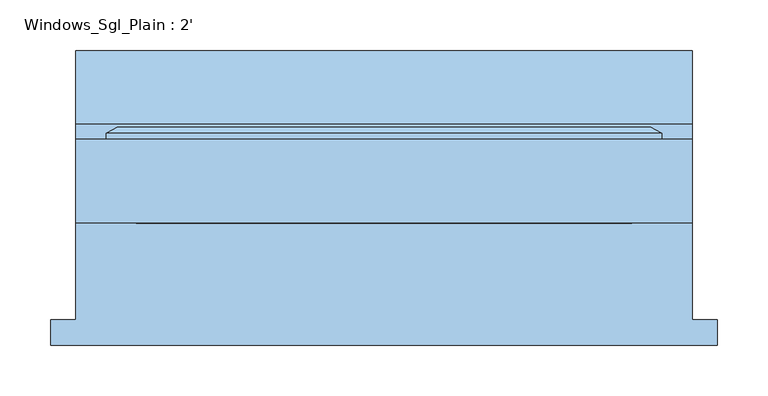
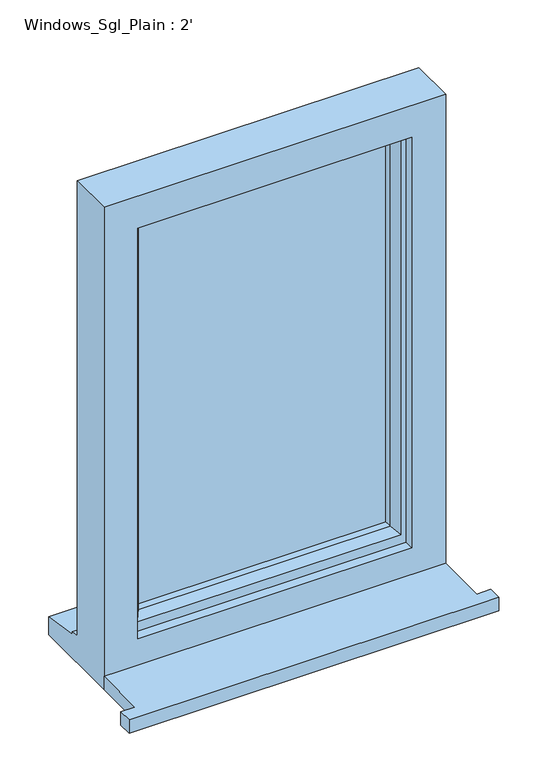
"""IFC4 building model written with IfcOpenShell, lengths in millimetres: window geometry, Windows_Sgl_Plain : 2'."""

from ifc_helpers import new_model, si_unit, frame, origin, place, context, project, spatial, polyline, outline, extrude, faceted_brep, source, transform, mapped, element, save


def windows_sgl_plain_2_8d1346b0(model_context):
    return source(origin(), model_context, "Body", "SolidModel", [
        extrude(outline(polyline([(-329.8, -130.8434322), (-329.8, -105.8434322), (-304.8, -105.8434322), (-304.8, -10.2434322), (304.8, -10.2434322), (304.8, -105.8434322), (329.8, -105.8434322), (329.8, -130.8434322), (-329.8, -130.8434322)])), frame((0.0, 0.0, 1200.0), z_axis=(0.0, 0.0, 1.0), x_axis=(1.0, 0.0, 0.0)), (0.0, 0.0, 1.0), 25.0),
        faceted_brep([(-304.8, -10.2434322, 1200.0), (304.8, -10.2434322, 1200.0), (304.8, -10.2434322, 2110.0), (-304.8, -10.2434322, 2110.0), (-244.8, -10.2434322, 2050.0), (244.8, -10.2434322, 2050.0), (244.8, -10.2434322, 1275.0), (-244.8, -10.2434322, 1275.0), (-304.8, 72.7565678, 2110.0), (-304.8, 72.7565678, 1251.0), (-304.8, 87.7565678, 1249.68767), (-304.8, 87.7565678, 1244.7449676), (-304.8, 160.2565678, 1233.8088847), (-304.8, 160.2565678, 1200.0), (304.8, 72.7565678, 2110.0), (304.8, 72.7565678, 1251.0), (-264.8, 72.7565678, 2070.0), (-264.8, 72.7565678, 1263.0), (264.8, 72.7565678, 1263.0), (264.8, 72.7565678, 2070.0), (-264.8, 7.7565678, 2070.0), (-264.8, 7.7565678, 1263.0), (264.8, 7.7565678, 2070.0), (264.8, 7.7565678, 1263.0), (-244.8, 7.7565678, 2050.0), (-244.8, 7.7565678, 1275.0), (244.8, 7.7565678, 1275.0), (244.8, 7.7565678, 2050.0), (304.8, 160.2565678, 1200.0), (304.8, 160.2565678, 1233.8088847), (304.8, 87.7565678, 1244.7449676), (304.8, 87.7565678, 1249.68767)], [[[0, 1, 2, 3], [4, 5, 6, 7]], [[0, 3, 8, 9, 10, 11, 12, 13]], [[9, 8, 14, 15], [16, 17, 18, 19]], [[17, 16, 20, 21]], [[20, 22, 23, 21], [24, 25, 26, 27]], [[24, 4, 7, 25]], [[3, 2, 14, 8]], [[16, 19, 22, 20]], [[5, 4, 24, 27]], [[15, 14, 2, 1, 28, 29, 30, 31]], [[19, 18, 23, 22]], [[5, 27, 26, 6]], [[28, 1, 0, 13]], [[29, 28, 13, 12]], [[30, 29, 12, 11]], [[31, 30, 11, 10]], [[15, 31, 10, 9]], [[21, 23, 18, 17]], [[7, 6, 26, 25]]]),
        extrude(outline(polyline([(234.8, 36.7565678), (-234.8, 36.7565678), (-234.8, 60.7565678), (234.8, 60.7565678), (234.8, 36.7565678)])), frame((0.0, 0.0, 1293.0), z_axis=(0.0, 0.0, 1.0), x_axis=(1.0, 0.0, 0.0)), (0.0, 0.0, 1.0), 747.0),
        faceted_brep([(-274.8, 72.7565678, 2080.0), (-274.8, 78.5300705, 2080.0), (-274.8, 78.5300705, 1253.0), (-274.8, 72.7565678, 1253.0), (-264.8, 7.7565678, 2070.0), (-264.8, 72.7565678, 2070.0), (-264.8, 72.7565678, 1263.0), (-264.8, 7.7565678, 1263.0), (-224.8, 22.2494677, 2030.0), (-234.9480377, 7.7565678, 2040.1480377), (-234.9480377, 7.7565678, 1292.8519623), (-224.8, 22.2494677, 1303.0), (-224.8, 36.7565678, 2030.0), (-224.8, 36.7565678, 1303.0), (-234.8, 60.7565678, 2040.0), (-234.8, 36.7565678, 2040.0), (-234.8, 36.7565678, 1293.0), (-234.8, 60.7565678, 1293.0), (-224.8, 78.5300705, 2030.0), (-224.8, 60.7565678, 2030.0), (-224.8, 60.7565678, 1303.0), (-224.8, 78.5300705, 1303.0), (-242.2457548, 84.3035732, 2047.4457548), (-242.2457548, 84.3035732, 1285.5542452), (-264.0153903, 84.3035732, 2069.2153903), (-264.0153903, 84.3035732, 1263.7846097), (274.8, 78.5300705, 1253.0), (274.8, 72.7565678, 1253.0), (264.8, 72.7565678, 1263.0), (264.8, 7.7565678, 1263.0), (234.9480377, 7.7565678, 1292.8519623), (224.8, 22.2494677, 1303.0), (224.8, 36.7565678, 1303.0), (234.8, 36.7565678, 1293.0), (234.8, 60.7565678, 1293.0), (224.8, 60.7565678, 1303.0), (224.8, 78.5300705, 1303.0), (242.2457548, 84.3035732, 1285.5542452), (264.0153903, 84.3035732, 1263.7846097), (274.8, 78.5300705, 2080.0), (274.8, 72.7565678, 2080.0), (264.8, 72.7565678, 2070.0), (264.8, 7.7565678, 2070.0), (234.9480377, 7.7565678, 2040.1480377), (224.8, 22.2494677, 2030.0), (224.8, 36.7565678, 2030.0), (234.8, 36.7565678, 2040.0), (234.8, 60.7565678, 2040.0), (224.8, 60.7565678, 2030.0), (224.8, 78.5300705, 2030.0), (242.2457548, 84.3035732, 2047.4457548), (264.0153903, 84.3035732, 2069.2153903)], [[[0, 1, 2, 3]], [[4, 5, 6, 7]], [[8, 9, 10, 11]], [[12, 8, 11, 13]], [[14, 15, 16, 17]], [[18, 19, 20, 21]], [[22, 18, 21, 23]], [[1, 24, 25, 2]], [[3, 2, 26, 27]], [[7, 6, 28, 29]], [[11, 10, 30, 31]], [[13, 11, 31, 32]], [[17, 16, 33, 34]], [[21, 20, 35, 36]], [[23, 21, 36, 37]], [[2, 25, 38, 26]], [[27, 26, 39, 40]], [[29, 28, 41, 42]], [[31, 30, 43, 44]], [[32, 31, 44, 45]], [[34, 33, 46, 47]], [[36, 35, 48, 49]], [[37, 36, 49, 50]], [[26, 38, 51, 39]], [[40, 39, 1, 0]], [[3, 27, 40, 0], [5, 41, 28, 6]], [[42, 41, 5, 4]], [[7, 29, 42, 4], [9, 43, 30, 10]], [[44, 43, 9, 8]], [[45, 44, 8, 12]], [[15, 46, 33, 16], [13, 32, 45, 12]], [[47, 46, 15, 14]], [[17, 34, 47, 14], [19, 48, 35, 20]], [[49, 48, 19, 18]], [[50, 49, 18, 22]], [[24, 51, 38, 25], [23, 37, 50, 22]], [[39, 51, 24, 1]]]),
    ])


if __name__ == "__main__":
    model = new_model("IFC4")
    model_context = context("Model", 3, world=origin())
    ifc_project = project(units=[si_unit("LENGTHUNIT", "METRE", prefix="MILLI")], contexts=[model_context])
    site = spatial("IfcSite", under=ifc_project)
    building = spatial("IfcBuilding", under=site)
    placement = place(None, origin())
    windows_sgl_plain_2_shape = windows_sgl_plain_2_8d1346b0(model_context)
    element("IfcWindow", 1, ObjectType="Windows_Sgl_Plain : 2'", at=placement, inside=building, context=model_context, shape_type="MappedRepresentation", body=[
        mapped(windows_sgl_plain_2_shape, transform((0.0, 0.0, 0.0), x_axis=(1.0, 0.0, 0.0), y_axis=(0.0, 1.0, 0.0), z_axis=(0.0, 0.0, 1.0))),
    ])
    save(model, "model.ifc")

# Revit data of these elements
# Type "Windows_Sgl_Plain : 2'"
#   Type Mark = "64"
#   Operation = "SinglePanel"
#   Construction Type Id = "SGL"
#   Manufacturer = "Revit"
#   Keynote = "L10"
#   Analytic Construction = "Large single-glazed windows"
#   Wrap Layers (Ext) from Ext = 0' - 4.03543"
#   Wrap Layers (Int) from Ext = 0' - 6.98819"
#   Window Board Projection = 0' - 0.98425"
#   Window Board Extension = 0' - 0.98425"
#   Visual Light Transmittance = 0.9
#   Solar Heat Gain Coefficient = 0.86
#   Rough Width = 2' - 0"
#   Rough Height = 2' - 11.82677"
#   Height = 2' - 11.82677"
#   Width = 2' - 0"
#   Heat Transfer Coefficient (U) = 5.5617 W/(m²·K)
#   Glazing Thickness = 0' - 0.94488"
#   FrameOffset - External = 0' - 1.9685"
#   Frame Depth = 0' - 2.55906"
#   Default Head Height = 6' - 11.07087"
#   Cill Depth = 0' - 3.44488"
#   Cavity Closer Width = 0' - 1.9685"
#   Cavity Closer Offset from Ext = 0' - 4.03543"
#   Cavity Closer Depth = 0' - 3.34646"
#   Vis - Cavity Closers = yes
#   Define Thermal Properties by = 1
#   Material Trim = Window Frame
#   Material Glass = Glass
#   Material Frame = Window Frame
#   Wall Closure = (empty or 0)
# Element 1 (IfcWindow, "Windows_Sgl_Plain : 2'")
#   Materials on its faces: "Window Frame", "Glass"
# Materials
#   "Window Frame": colour RGB 249 249 249, transparency 0, Keynote = "L10", Cost = 0
#   "Glass": class "Glass", colour RGB 0 128 192, transparency 0.9, Description = "Soda Lime Glass", Cost = 0
